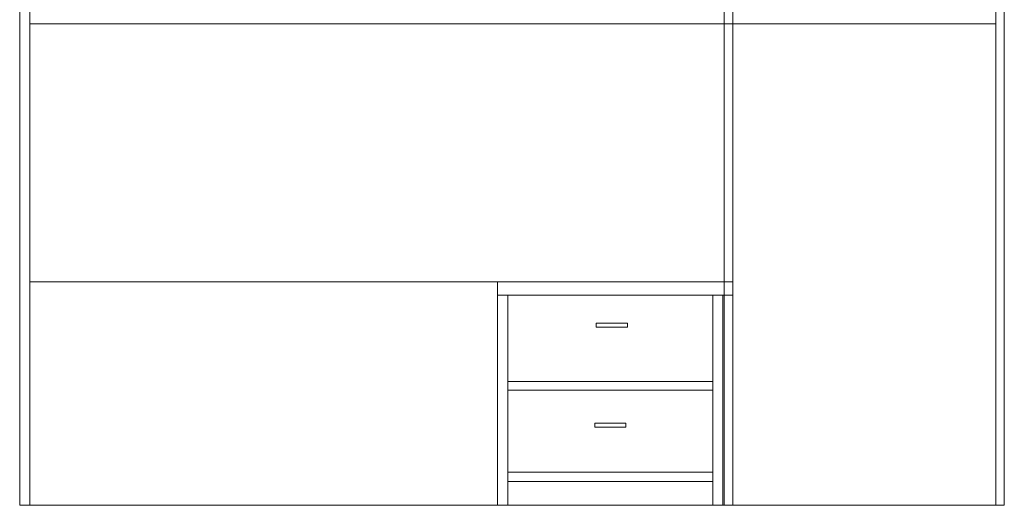
# Model space of a CAD drawing. Units: inches. Extents: x -17 to 1735, y -531 to 60.
# Tile 6 of 27: x 1734.65811 to 1734.73921, y -150.26454 to -150.22453. Entities that reach past the tile are written whole.
import ezdxf

# ---------------------------------------------------------------- set-up
doc = ezdxf.new("R2010")
doc.units = ezdxf.units.IN
doc.header["$MEASUREMENT"] = 0
doc.layers.add('A-FURN', color=242, linetype='Continuous', lineweight=18, true_color=0xcd2027)

# ---------------------------------------------------------------- blocks, each defined once
blk = doc.blocks.new('childrens_room_2')
for p, q in [((69.7359, 55.4342), (69.7359, 52.9342)), ((69.7569, 55.4342), (69.7569, 52.9342)), ((71.7779, 55.4342), (71.7779, 52.9342)), ((71.7959, 55.4342), (71.7959, 52.9342)), ((71.2099, 52.9342), (71.2099, 55.3342)), ((71.2279, 52.9342), (71.2279, 55.3342)), ((69.7569, 53.9414), (71.7779, 53.9414)), ((69.7569, 53.4019), (71.2279, 53.4019)), ((70.7359, 53.4019), (70.7359, 53.3736)), ((71.2279, 53.3736), (71.2279, 53.4019)), ((70.7359, 53.3736), (70.7359, 52.9342)), ((70.7359, 53.3736), (71.2279, 53.3736)), ((70.7359, 53.3736), (70.7359, 52.9342)), ((70.7569, 53.3736), (70.7569, 52.9342)), ((71.1859, 53.3736), (71.1859, 52.9342)), ((71.2069, 53.3736), (71.2069, 52.9342)), ((70.7569, 53.1931), (71.1859, 53.1931)), ((70.7569, 53.1751), (71.1859, 53.1751)), ((70.7569, 53.0037), (71.1859, 53.0037)), ((70.7569, 52.9837), (71.1859, 52.9837)), ((69.7359, 52.9342), (71.7959, 52.9342))]:
    blk.add_line(p, q)
for points in [[(71.0073, 53.3153), (70.9422, 53.3153), (70.9422, 53.3073), (71.0073, 53.3073)], [(71.0041, 53.1058), (70.939, 53.1058), (70.939, 53.0978), (71.0041, 53.0978)]]:
    blk.add_lwpolyline(points, close=True)

msp = doc.modelspace()

# ---------------------------------------------------------------- block references
at = {"layer": 'A-FURN', "xscale": 0.0393700787401575, "yscale": 0.0393700787401575, "zscale": 0.0393700787401575}
msp.add_blockref('childrens_room_2', (1731.912601, -152.348565), dxfattribs=at)

doc.saveas('drawing.dxf')
